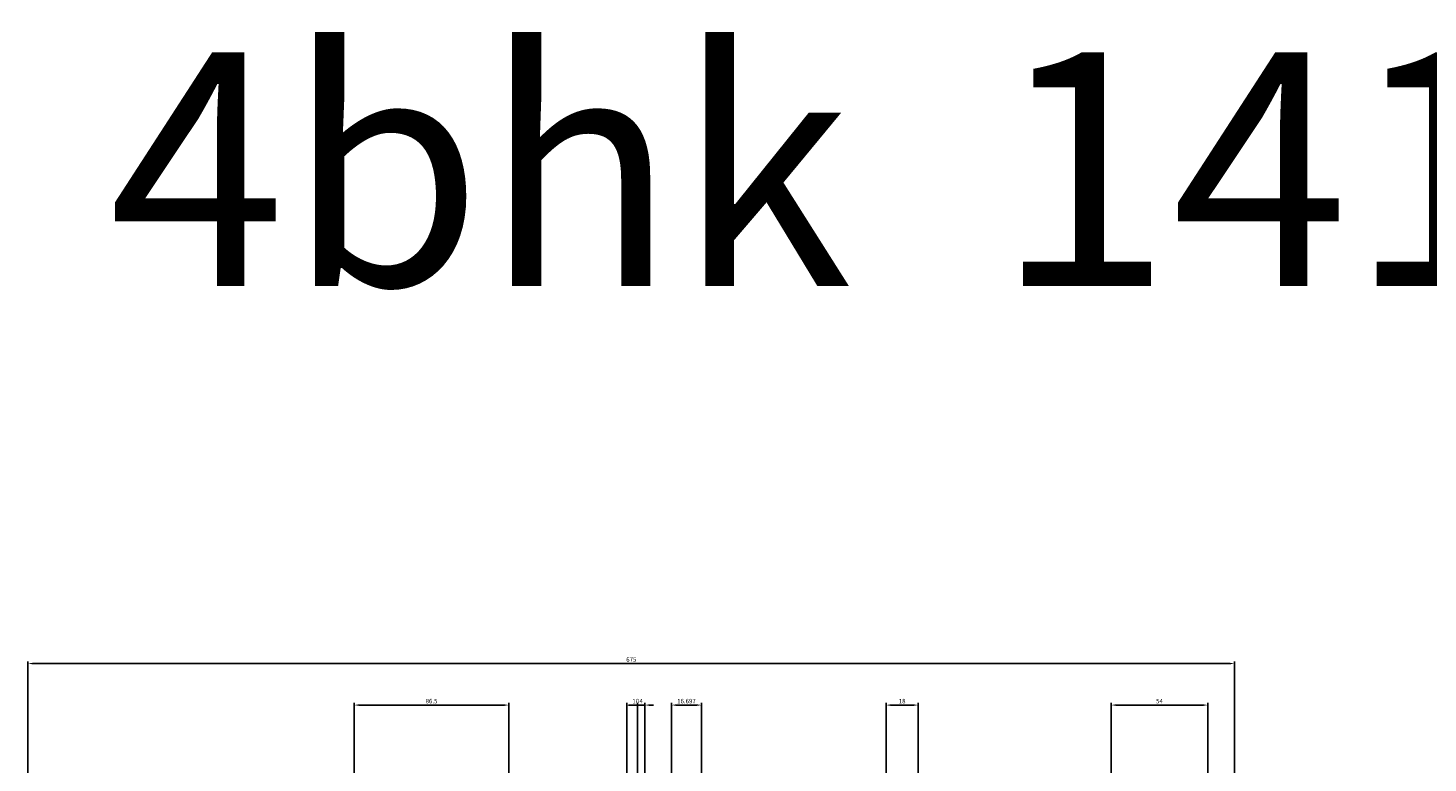
# Model space of a CAD drawing. Units: inches. Extents: x 604 to 3492, y -123 to 1737.
# Tile 11 of 20: x 678 to 1461, y 1326 to 1737. Entities that reach past the tile are written whole.
import ezdxf

# ---------------------------------------------------------------- set-up
doc = ezdxf.new("R2010")
doc.units = ezdxf.units.IN
doc.layers.add('A-ANNO-DIMS', color=2, linetype='Continuous', lineweight=18)
doc.layers.add('A-ANNO-TEXT', color=7, linetype='Continuous', lineweight=35)
doc.styles.get("Standard").update_dxf_attribs({"font": 'arial.ttf'})
doc.dimstyles.new('ISO-25', dxfattribs={"dimtxt": 2.5, "dimasz": 2.5, "dimexe": 1.25, "dimexo": 0.625, "dimtad": 1, "dimtxsty": 'Standard', "dimcen": 2.5, "dimadec": 0, "dimazin": 0, "dimtfac": 1, "dimtmove": 0, "dimatfit": 3, "dimfxl": 1, "dimarcsym": 0})

# ---------------------------------------------------------------- blocks, each defined once
blk = doc.blocks.new('*D13')
at = {"layer": 'A-ANNO-DIMS', "color": 0, "lineweight": -2, "transparency": 16777216}
for p, q in [((678.01, 1288.33), (678.01, 1383.12)), ((680.51, 1381.87), (1350.51, 1381.87)), ((1353.01, 1288.33), (1353.01, 1383.12))]:
    blk.add_line(p, q, dxfattribs=at)
at = {"layer": 'A-ANNO-DIMS', "color": 0, "transparency": 16777216}
for points in [[(680.51, 1382.29), (680.51, 1381.46), (678.01, 1381.87)], [(1350.51, 1382.29), (1350.51, 1381.46), (1353.01, 1381.87)]]:
    blk.add_solid(points, dxfattribs=at)
at = {"layer": 'Defpoints', "color": 0, "transparency": 16777216}
for p in [(1353.01, 1381.87), (678.01, 1287.7), (1353.01, 1287.7)]:
    blk.add_point(p, dxfattribs=at)
at = {"layer": 'A-ANNO-DIMS', "color": 0, "transparency": 16777216, "insert": (1015.51, 1383.78), "char_height": 2.5, "attachment_point": 5}
blk.add_mtext('675', dxfattribs=at)
blk = doc.blocks.new('*D90')
at = {"layer": 'A-ANNO-DIMS', "color": 0, "lineweight": -2, "transparency": 16777216}
for p, q in [((1016.51, 1358.65), (1014.01, 1358.65)), ((1019.01, 423.33), (1019.01, 1359.9)), ((1023.01, 1358.65), (1019.01, 1358.65)), ((1023.01, 423.33), (1023.01, 1359.9)), ((1025.51, 1358.65), (1028.01, 1358.65))]:
    blk.add_line(p, q, dxfattribs=at)
at = {"layer": 'A-ANNO-DIMS', "color": 0, "transparency": 16777216}
for points in [[(1016.51, 1359.07), (1016.51, 1358.23), (1019.01, 1358.65)], [(1025.51, 1359.07), (1025.51, 1358.23), (1023.01, 1358.65)]]:
    blk.add_solid(points, dxfattribs=at)
at = {"layer": 'Defpoints', "color": 0, "transparency": 16777216}
for p in [(1019.01, 1358.65), (1019.01, 422.7), (1023.01, 422.7)]:
    blk.add_point(p, dxfattribs=at)
at = {"layer": 'A-ANNO-DIMS', "color": 0, "transparency": 16777216, "insert": (1021.01, 1360.53), "char_height": 2.5, "attachment_point": 5}
blk.add_mtext('4', dxfattribs=at)
blk = doc.blocks.new('*D91')
at = {"layer": 'A-ANNO-DIMS', "color": 0, "lineweight": -2, "transparency": 16777216}
for p, q in [((860.51, 408.33), (860.51, 1359.9)), ((863.01, 1358.65), (944.51, 1358.65)), ((947.01, 408.33), (947.01, 1359.9))]:
    blk.add_line(p, q, dxfattribs=at)
at = {"layer": 'A-ANNO-DIMS', "color": 0, "transparency": 16777216}
for points in [[(863.01, 1359.07), (863.01, 1358.23), (860.51, 1358.65)], [(944.51, 1359.07), (944.51, 1358.23), (947.01, 1358.65)]]:
    blk.add_solid(points, dxfattribs=at)
at = {"layer": 'Defpoints', "color": 0, "transparency": 16777216}
for p in [(947.01, 1358.65), (860.51, 407.7), (947.01, 407.7)]:
    blk.add_point(p, dxfattribs=at)
at = {"layer": 'A-ANNO-DIMS', "color": 0, "transparency": 16777216, "insert": (903.76, 1360.55), "char_height": 2.5, "attachment_point": 5}
blk.add_mtext('86.5', dxfattribs=at)
blk = doc.blocks.new('*D93')
at = {"layer": 'A-ANNO-DIMS', "color": 0, "lineweight": -2, "transparency": 16777216}
for p, q in [((1038.01, 588.33), (1038.01, 1359.9)), ((1040.51, 1358.65), (1052.21, 1358.65)), ((1054.71, 588.27), (1054.71, 1359.9))]:
    blk.add_line(p, q, dxfattribs=at)
at = {"layer": 'A-ANNO-DIMS', "color": 0, "transparency": 16777216}
for points in [[(1040.51, 1359.07), (1040.51, 1358.23), (1038.01, 1358.65)], [(1052.21, 1359.07), (1052.21, 1358.23), (1054.71, 1358.65)]]:
    blk.add_solid(points, dxfattribs=at)
at = {"layer": 'Defpoints', "color": 0, "transparency": 16777216}
for p in [(1054.71, 1358.65), (1038.01, 587.7), (1054.71, 587.64)]:
    blk.add_point(p, dxfattribs=at)
at = {"layer": 'A-ANNO-DIMS', "color": 0, "transparency": 16777216, "insert": (1046.36, 1360.55), "char_height": 2.5, "attachment_point": 5}
blk.add_mtext('16.697', dxfattribs=at)
blk = doc.blocks.new('*D95')
at = {"layer": 'A-ANNO-DIMS', "color": 0, "lineweight": -2, "transparency": 16777216}
for p, q in [((1284.01, 740.33), (1284.01, 1359.9)), ((1286.51, 1358.65), (1335.51, 1358.65)), ((1338.01, 740.33), (1338.01, 1359.9))]:
    blk.add_line(p, q, dxfattribs=at)
at = {"layer": 'A-ANNO-DIMS', "color": 0, "transparency": 16777216}
for points in [[(1286.51, 1359.07), (1286.51, 1358.23), (1284.01, 1358.65)], [(1335.51, 1359.07), (1335.51, 1358.23), (1338.01, 1358.65)]]:
    blk.add_solid(points, dxfattribs=at)
at = {"layer": 'Defpoints', "color": 0, "transparency": 16777216}
for p in [(1338.01, 1358.65), (1284.01, 739.7), (1338.01, 739.7)]:
    blk.add_point(p, dxfattribs=at)
at = {"layer": 'A-ANNO-DIMS', "color": 0, "transparency": 16777216, "insert": (1311.01, 1360.55), "char_height": 2.5, "attachment_point": 5}
blk.add_mtext('54', dxfattribs=at)
blk = doc.blocks.new('*D96')
at = {"layer": 'A-ANNO-DIMS', "color": 0, "lineweight": -2, "transparency": 16777216}
for p, q in [((1158.01, 740.33), (1158.01, 1359.9)), ((1160.51, 1358.65), (1173.51, 1358.65)), ((1176.01, 740.33), (1176.01, 1359.9))]:
    blk.add_line(p, q, dxfattribs=at)
at = {"layer": 'A-ANNO-DIMS', "color": 0, "transparency": 16777216}
for points in [[(1160.51, 1359.07), (1160.51, 1358.23), (1158.01, 1358.65)], [(1173.51, 1359.07), (1173.51, 1358.23), (1176.01, 1358.65)]]:
    blk.add_solid(points, dxfattribs=at)
at = {"layer": 'Defpoints', "color": 0, "transparency": 16777216}
for p in [(1176.01, 1358.65), (1158.01, 739.7), (1176.01, 739.7)]:
    blk.add_point(p, dxfattribs=at)
at = {"layer": 'A-ANNO-DIMS', "color": 0, "transparency": 16777216, "insert": (1167.01, 1360.55), "char_height": 2.5, "attachment_point": 5}
blk.add_mtext('18', dxfattribs=at)
blk = doc.blocks.new('*D99')
at = {"layer": 'A-ANNO-DIMS', "color": 0, "lineweight": -2, "transparency": 16777216}
for p, q in [((1013.01, 898.33), (1013.01, 1359.9)), ((1015.51, 1358.65), (1020.51, 1358.65)), ((1023.01, 913.33), (1023.01, 1359.9))]:
    blk.add_line(p, q, dxfattribs=at)
at = {"layer": 'A-ANNO-DIMS', "color": 0, "transparency": 16777216}
for points in [[(1015.51, 1359.07), (1015.51, 1358.23), (1013.01, 1358.65)], [(1020.51, 1359.07), (1020.51, 1358.23), (1023.01, 1358.65)]]:
    blk.add_solid(points, dxfattribs=at)
at = {"layer": 'Defpoints', "color": 0, "transparency": 16777216}
for p in [(1023.01, 1358.65), (1023.01, 912.7), (1013.01, 897.7)]:
    blk.add_point(p, dxfattribs=at)
at = {"layer": 'A-ANNO-DIMS', "color": 0, "transparency": 16777216, "insert": (1018.01, 1360.55), "char_height": 2.5, "attachment_point": 5}
blk.add_mtext('10', dxfattribs=at)

msp = doc.modelspace()

# ---------------------------------------------------------------- texts
at = {"layer": 'A-ANNO-TEXT'}
msp.add_text('4bhk  1415sq ft', height=130.709805, dxfattribs=at).set_placement((723.1092, 1593.2028))

# ---------------------------------------------------------------- dimensions: what is measured, and where the dimension line sits
at = {"layer": 'A-ANNO-DIMS'}
for base, p1, p2, override, picture, middle in [((1353.0111, 1381.8744), (678.0111, 1287.7004), (1353.0111, 1287.7004), {"dimclrd": 0, "dimclre": 0, "dimclrt": 0}, '*D13', (1015.5111, 1383.7759)), ((947.0111, 1358.6504), (860.5111, 407.7004), (947.0111, 407.7004), {"dimdec": 1, "dimlfac": 1, "dimrnd": 0, "dimzin": 0, "dimdsep": 46, "dimlunit": 2}, '*D91', (903.7611, 1360.5519)), ((1023.0111, 1358.6504), (1013.0111, 897.7004), (1023.0111, 912.7004), {"dimdec": 0, "dimlfac": 1, "dimrnd": 0, "dimzin": 0, "dimdsep": 46, "dimlunit": 2}, '*D99', (1018.0111, 1360.5519)), ((1019.0111, 1358.6504), (1023.0111, 422.7004), (1019.0111, 422.7004), {"dimdec": 0, "dimlfac": 1, "dimrnd": 0, "dimzin": 0, "dimdsep": 46, "dimlunit": 2}, '*D90', (1021.0111, 1360.5254)), ((1054.7083, 1358.6504), (1038.0111, 587.7004), (1054.7083, 587.6435), {"dimdec": 3, "dimlfac": 1, "dimrnd": 0, "dimzin": 0, "dimdsep": 46, "dimlunit": 2}, '*D93', (1046.3597, 1360.5519)), ((1176.0111, 1358.6504), (1158.0111, 739.7004), (1176.0111, 739.7004), {"dimdec": 0, "dimlfac": 1, "dimrnd": 0, "dimzin": 0, "dimdsep": 46, "dimlunit": 2}, '*D96', (1167.0111, 1360.5519)), ((1338.0111, 1358.6504), (1284.0111, 739.7004), (1338.0111, 739.7004), {"dimdec": 0, "dimlfac": 1, "dimrnd": 0, "dimzin": 0, "dimdsep": 46, "dimlunit": 2}, '*D95', (1311.0111, 1360.5468))]:
    dim = msp.add_linear_dim(base=base, p1=p1, p2=p2, dimstyle='ISO-25', override=override, dxfattribs=at)
    dim.commit()
    dim.dimension.update_dxf_attribs({"geometry": picture, "text_midpoint": middle})

doc.saveas('drawing.dxf')
